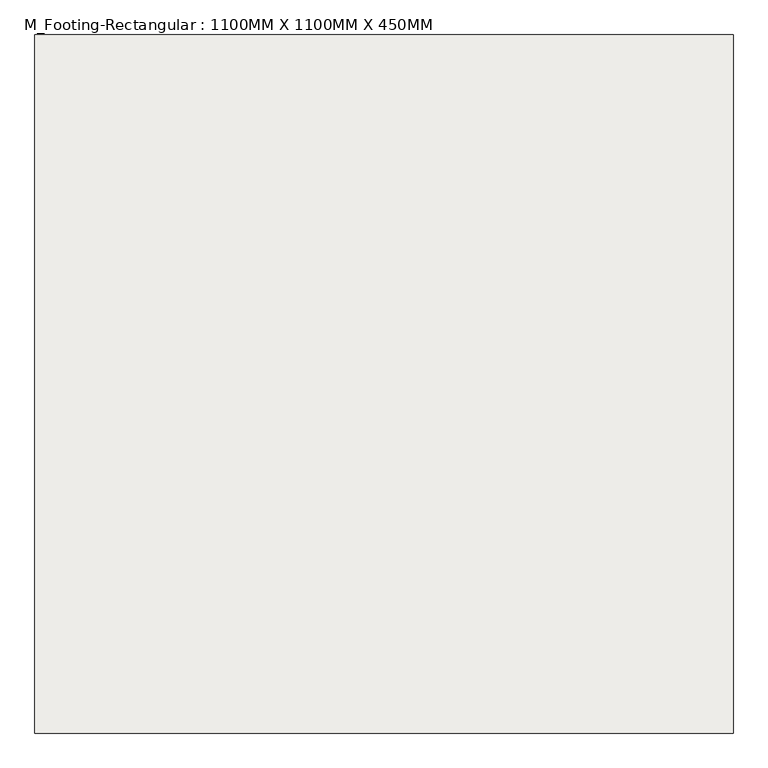
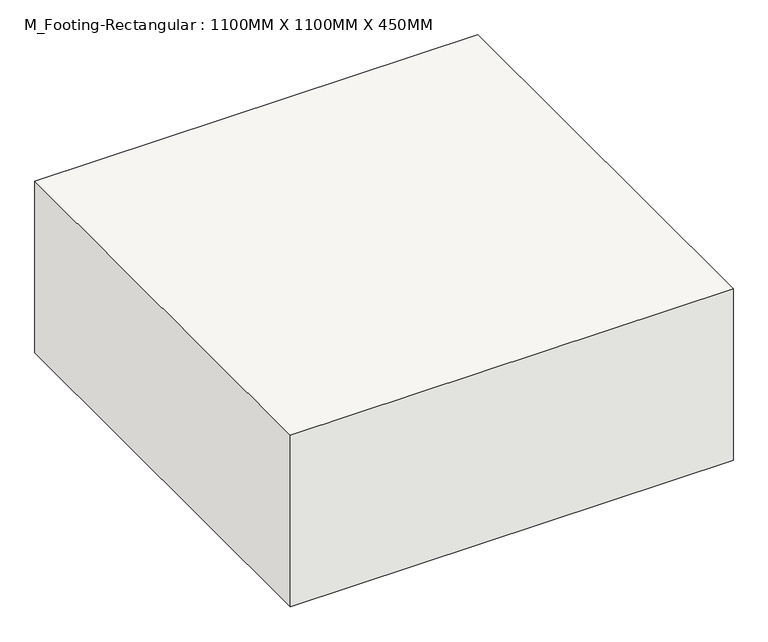
"""IFC4 building model written with IfcOpenShell, lengths in millimetres: slab geometry, M_Footing-Rectangular : 1100MM X 1100MM X 450MM."""

from ifc_helpers import new_model, si_unit, frame, origin, place, context, project, spatial, polyline, outline, extrude, source, transform, mapped, element, save


def m_footing_rectangular_1100mm_x_1100mm_x_450mm_64323a20(model_context):
    return source(origin(), model_context, "Body", "SweptSolid", [
        extrude(outline(polyline([(550.0, 550.0), (550.0, -550.0), (-550.0, -550.0), (-550.0, 550.0), (550.0, 550.0)])), frame((0.0, 0.0, -450.0), z_axis=(0.0, 0.0, 1.0), x_axis=(1.0, 0.0, 0.0)), (0.0, 0.0, 1.0), 450.0),
    ])


if __name__ == "__main__":
    model = new_model("IFC4")
    model_context = context("Model", 3, world=origin())
    ifc_project = project(units=[si_unit("LENGTHUNIT", "METRE", prefix="MILLI")], contexts=[model_context])
    site = spatial("IfcSite", under=ifc_project)
    building = spatial("IfcBuilding", under=site)
    placement = place(None, origin())
    m_footing_rectangular_1100mm_x_1100mm_x_450mm_shape = m_footing_rectangular_1100mm_x_1100mm_x_450mm_64323a20(model_context)
    element("IfcSlab", 1, ObjectType="M_Footing-Rectangular : 1100MM X 1100MM X 450MM", at=placement, inside=building, context=model_context, shape_type="MappedRepresentation", body=[
        mapped(m_footing_rectangular_1100mm_x_1100mm_x_450mm_shape, transform((0.0, 0.0, 0.0), x_axis=(1.0, 0.0, 0.0), y_axis=(0.0, 1.0, 0.0), z_axis=(0.0, 0.0, 1.0))),
    ])
    save(model, "model.ifc")

# Revit data of these elements
# Type "M_Footing-Rectangular : 1100MM X 1100MM X 450MM"
#   Width = 1100 mm
#   Length = 1100 mm
#   Foundation Thickness = 450 mm
#   Structural Material [instance default] = Concrete, Cast-in-Place gray
#   Assembly Code = ""
# Element 1 (IfcSlab, "M_Footing-Rectangular : 1100MM X 1100MM X 450MM")
#   Materials on its faces: "Concrete, Cast-in-Place gray"
# Materials
#   "Concrete, Cast-in-Place gray": class "Concrete", colour RGB 192 192 192, transparency 0, Description = "Cast-in-place concrete", Cost = 0
